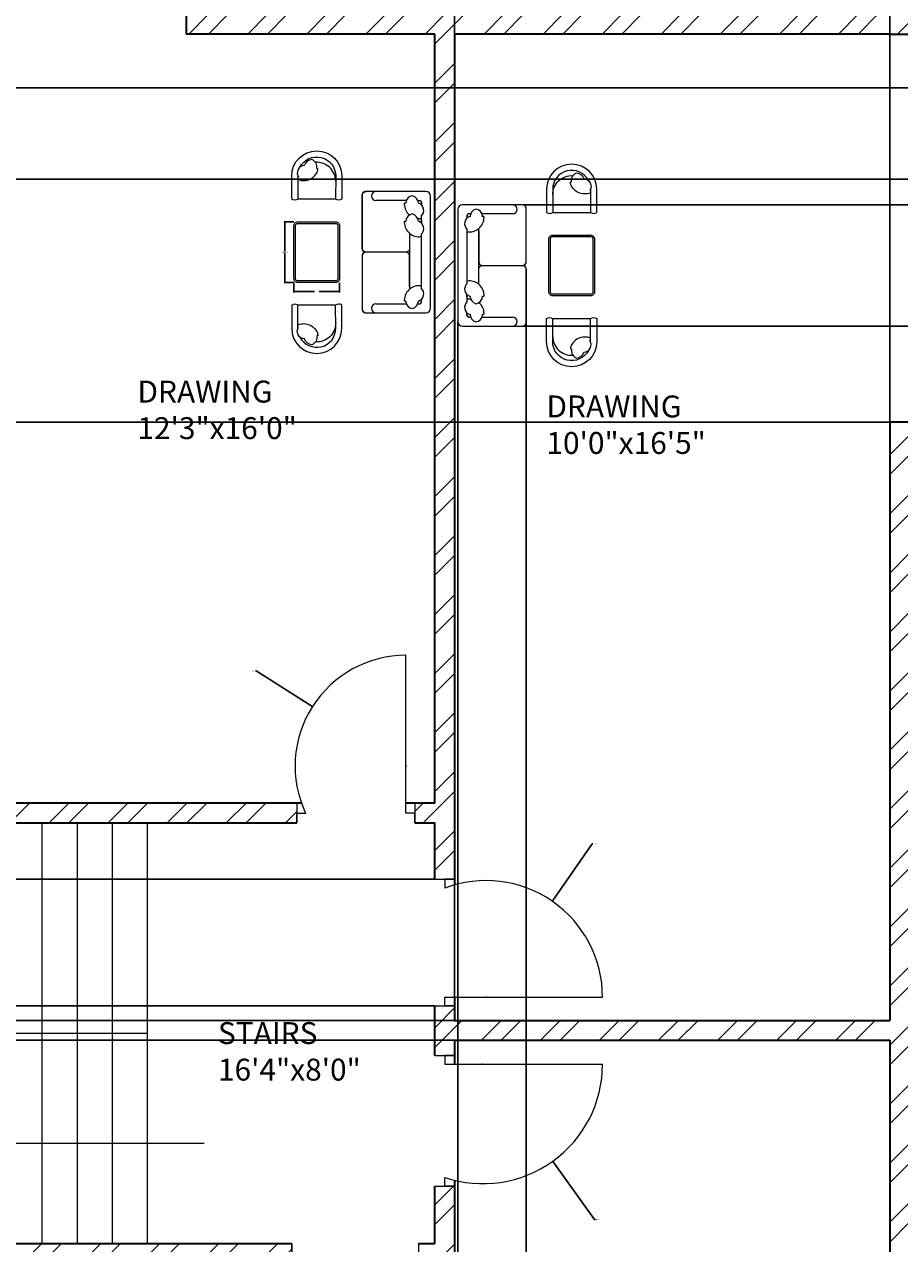
# Model space of a CAD drawing. Units: inches. Extents: x 2008 to 2657, y 1077 to 2165.
# Tile 9 of 16: x 2209 to 2409, y 1567 to 1845. Entities that reach past the tile are written whole.
import ezdxf

# ---------------------------------------------------------------- set-up
doc = ezdxf.new("R2010")
doc.units = ezdxf.units.IN
for name, color, linetype, lineweight in [('A-ANNO-DIMS', 2, 'Continuous', 18), ('A-AREA-IDEN', 4, 'Continuous', 18), ('A-DOOR', 11, 'Continuous', 18), ('A-FLOR-STRS', 60, 'Continuous', 18), ('A-FURN', 8, 'Continuous', 13), ('A-WALL', 7, 'Continuous', 35)]:
    doc.layers.add(name, color=color, linetype=linetype, lineweight=lineweight)
doc.layers.add('A-WALL-PATT', color=30, linetype='Continuous', lineweight=13, true_color=0xf8991e)
doc.styles.get("Standard").update_dxf_attribs({"font": 'arial.ttf'})
doc.dimstyles.get("Standard").update_dxf_attribs({"dimtxt": 0.18, "dimasz": 0.18, "dimexe": 0.18, "dimexo": 0.0625, "dimgap": 0.09, "dimtad": 0, "dimtih": 1, "dimtoh": 1, "dimdec": 4, "dimzin": 0, "dimdsep": 46, "dimtxsty": 'Standard', "dimcen": 0.09, "dimadec": 0, "dimazin": 0, "dimtfac": 1, "dimtdec": 4, "dimtofl": 0, "dimtmove": 0, "dimatfit": 3, "dimfxl": 1, "dimtolj": 1, "dimtzin": 0, "dimarcsym": 0})

# ---------------------------------------------------------------- blocks, each defined once
blk = doc.blocks.new('A$C1352')
at = {"color": 0}
for points in [[(0.003, 0.053), (0.003, 0.553, -0.414214), (0.053, 0.603), (0.753, 0.603, -0.414214), (0.803, 0.553), (0.803, 0.053, -0.414214), (0.753, 0.003), (0.053, 0.003, -0.414214)], [(0.023, 0.053), (0.023, 0.553, -0.414214), (0.053, 0.583), (0.753, 0.583, -0.414214), (0.783, 0.553), (0.783, 0.053, -0.414214), (0.753, 0.023), (0.053, 0.023, -0.414214)]]:
    blk.add_lwpolyline(points, format="xyb", close=True, dxfattribs=at)
blk = doc.blocks.new('LOUNGE-CHAIR')
blk.add_line((1.39, 5.54), (1.38, 0.26))
at = {"ltscale": 0.03}
blk.add_lwpolyline([(1.38, 0.26, -0.369229), (0, 0.27), (0, 5.54, -1), (11.42, 5.53), (11.42, 0.25, -0.369229), (10.03, 0.26)], format="xyb", close=True, dxfattribs=at)
blk.add_lwpolyline([(1.88, 7.54, -0.785087), (10.04, 5.53), (10.03, 0.26)], format="xyb")
for centre, radius, start, end in [((4.77, 7.34), 1.95, 94.9999, 161.3534), ((3.98, 7.61), 1.78, 346.6403, 69.4695), ((5.71, 4.32), 4.33, 359.9461, 93.658), ((3.01, 6.23), 1.73, 92.9922, 214.1401), ((5.71, 5.54), 4.33, 178.8536, 179.9461), ((2.75, 7.82), 3.35, 247.0143, 344.2857), ((5.79, 7.01), 0.207, 330.6238, 113.7423)]:
    blk.add_arc(centre, radius, start, end)
blk = doc.blocks.new('*D17')
at = {"layer": 'A-ANNO-DIMS', "color": 0, "lineweight": -2, "transparency": 16777216}
for p, q in [((2270.8, 1799.92), (2268.61, 1799.92)), ((2268.79, 1799.74), (2268.79, 1793.18)), ((2268.79, 1786.26), (2268.79, 1792.82)), ((2270.8, 1786.08), (2268.61, 1786.08))]:
    blk.add_line(p, q, dxfattribs=at)
at = {"layer": 'A-ANNO-DIMS', "color": 0, "transparency": 16777216}
for points in [[(2268.76, 1799.74), (2268.82, 1799.74), (2268.79, 1799.92)], [(2268.76, 1786.26), (2268.82, 1786.26), (2268.79, 1786.08)]]:
    blk.add_solid(points, dxfattribs=at)
at = {"layer": 'Defpoints', "color": 0, "transparency": 16777216}
for p in [(2270.87, 1799.92), (2268.79, 1786.08), (2270.87, 1786.08)]:
    blk.add_point(p, dxfattribs=at)
at = {"layer": 'A-ANNO-DIMS', "color": 0, "transparency": 16777216, "insert": (2268.79, 1793), "char_height": 0.18, "attachment_point": 5}
blk.add_mtext('\\A1;TABLE 14 TYP.', dxfattribs=at)
blk = doc.blocks.new('*D18')
at = {"layer": 'A-ANNO-DIMS', "color": 0, "lineweight": -2, "transparency": 16777216}
for p, q in [((2270.87, 1786.01), (2270.87, 1783.82)), ((2271.05, 1784), (2275.54, 1784)), ((2281.07, 1784), (2276.58, 1784)), ((2281.25, 1786.01), (2281.25, 1783.82))]:
    blk.add_line(p, q, dxfattribs=at)
at = {"layer": 'A-ANNO-DIMS', "color": 0, "transparency": 16777216}
for points in [[(2271.05, 1784.03), (2271.05, 1783.97), (2270.87, 1784)], [(2281.07, 1784.03), (2281.07, 1783.97), (2281.25, 1784)]]:
    blk.add_solid(points, dxfattribs=at)
at = {"layer": 'Defpoints', "color": 0, "transparency": 16777216}
for p in [(2270.87, 1786.08), (2281.25, 1786.08), (2281.25, 1784)]:
    blk.add_point(p, dxfattribs=at)
at = {"layer": 'A-ANNO-DIMS', "color": 0, "transparency": 16777216, "insert": (2276.06, 1784), "char_height": 0.18, "attachment_point": 5}
blk.add_mtext('\\A1;10 TYP.', dxfattribs=at)
blk = doc.blocks.new('*D51')
at = {"layer": 'A-ANNO-DIMS', "color": 0, "lineweight": -2, "transparency": 16777216}
for p, q in [((2307.5, 1617.74), (2307.5, 2142.9)), ((2307.68, 2142.72), (2356.74, 2142.72)), ((2406.58, 2142.72), (2357.53, 2142.72)), ((2406.76, 1617.74), (2406.76, 2142.9))]:
    blk.add_line(p, q, dxfattribs=at)
at = {"layer": 'A-ANNO-DIMS', "color": 0, "transparency": 16777216}
for points in [[(2307.68, 2142.75), (2307.68, 2142.69), (2307.5, 2142.72)], [(2406.58, 2142.75), (2406.58, 2142.69), (2406.76, 2142.72)]]:
    blk.add_solid(points, dxfattribs=at)
at = {"layer": 'Defpoints', "color": 0, "transparency": 16777216}
for p in [(2406.76, 2142.72), (2307.5, 1617.67), (2406.76, 1617.67)]:
    blk.add_point(p, dxfattribs=at)
at = {"layer": 'A-ANNO-DIMS', "color": 0, "transparency": 16777216, "insert": (2357.13, 2142.72), "char_height": 0.18, "attachment_point": 5}
blk.add_mtext('\\A1;99.26', dxfattribs=at)
blk = doc.blocks.new('*D52')
at = {"layer": 'A-ANNO-DIMS', "color": 0, "lineweight": -2, "transparency": 16777216}
for p, q in [((2406.7, 1754.17), (2028.03, 1754.17)), ((2028.21, 1753.99), (2028.21, 1686.11)), ((2028.21, 1617.85), (2028.21, 1685.74)), ((2406.7, 1617.67), (2028.03, 1617.67))]:
    blk.add_line(p, q, dxfattribs=at)
at = {"layer": 'A-ANNO-DIMS', "color": 0, "transparency": 16777216}
for points in [[(2028.18, 1753.99), (2028.24, 1753.99), (2028.21, 1754.17)], [(2028.18, 1617.85), (2028.24, 1617.85), (2028.21, 1617.67)]]:
    blk.add_solid(points, dxfattribs=at)
at = {"layer": 'Defpoints', "color": 0, "transparency": 16777216}
for p in [(2406.76, 1754.17), (2028.21, 1617.67), (2406.76, 1617.67)]:
    blk.add_point(p, dxfattribs=at)
at = {"layer": 'A-ANNO-DIMS', "color": 0, "transparency": 16777216, "insert": (2028.21, 1685.92), "char_height": 0.18, "attachment_point": 5}
blk.add_mtext('\\A1;136.5', dxfattribs=at)
blk = doc.blocks.new('*D53')
at = {"layer": 'A-ANNO-DIMS', "color": 0, "lineweight": -2, "transparency": 16777216}
for p, q in [((2406.7, 1613.17), (2028.03, 1613.17)), ((2028.21, 1612.99), (2028.21, 1545.11)), ((2028.21, 1476.85), (2028.21, 1544.74)), ((2406.7, 1476.67), (2028.03, 1476.67))]:
    blk.add_line(p, q, dxfattribs=at)
at = {"layer": 'A-ANNO-DIMS', "color": 0, "transparency": 16777216}
for points in [[(2028.18, 1612.99), (2028.24, 1612.99), (2028.21, 1613.17)], [(2028.18, 1476.85), (2028.24, 1476.85), (2028.21, 1476.67)]]:
    blk.add_solid(points, dxfattribs=at)
at = {"layer": 'Defpoints', "color": 0, "transparency": 16777216}
for p in [(2406.76, 1613.17), (2028.21, 1476.67), (2406.76, 1476.67)]:
    blk.add_point(p, dxfattribs=at)
at = {"layer": 'A-ANNO-DIMS', "color": 0, "transparency": 16777216, "insert": (2028.21, 1544.92), "char_height": 0.18, "attachment_point": 5}
blk.add_mtext('\\A1;136.5', dxfattribs=at)
blk = doc.blocks.new('*D58')
at = {"layer": 'A-ANNO-DIMS', "color": 0, "lineweight": -2, "transparency": 16777216}
for p, q in [((2459.7, 1830.5), (2028.03, 1830.5)), ((2028.21, 1830.32), (2028.21, 1820.26)), ((2028.21, 1809.84), (2028.21, 1819.9)), ((2459.7, 1809.66), (2028.03, 1809.66))]:
    blk.add_line(p, q, dxfattribs=at)
at = {"layer": 'A-ANNO-DIMS', "color": 0, "transparency": 16777216}
for points in [[(2028.18, 1830.32), (2028.24, 1830.32), (2028.21, 1830.5)], [(2028.18, 1809.84), (2028.24, 1809.84), (2028.21, 1809.66)]]:
    blk.add_solid(points, dxfattribs=at)
at = {"layer": 'Defpoints', "color": 0, "transparency": 16777216}
for p in [(2028.21, 1830.5), (2459.76, 1830.5), (2459.76, 1809.66)]:
    blk.add_point(p, dxfattribs=at)
at = {"layer": 'A-ANNO-DIMS', "color": 0, "transparency": 16777216, "insert": (2028.21, 1820.08), "char_height": 0.18, "attachment_point": 5}
blk.add_mtext('\\A1;20.835', dxfattribs=at)
blk = doc.blocks.new('*D59')
at = {"layer": 'A-ANNO-DIMS', "color": 0, "lineweight": -2, "transparency": 16777216}
for p, q in [((2302.94, 1649.88), (2028.03, 1649.88)), ((2028.21, 1649.7), (2028.21, 1635.62)), ((2028.21, 1621.18), (2028.21, 1635.26)), ((2302.94, 1621), (2028.03, 1621))]:
    blk.add_line(p, q, dxfattribs=at)
at = {"layer": 'A-ANNO-DIMS', "color": 0, "transparency": 16777216}
for points in [[(2028.18, 1649.7), (2028.24, 1649.7), (2028.21, 1649.88)], [(2028.18, 1621.18), (2028.24, 1621.18), (2028.21, 1621)]]:
    blk.add_solid(points, dxfattribs=at)
at = {"layer": 'Defpoints', "color": 0, "transparency": 16777216}
for p in [(2028.21, 1649.88), (2303, 1649.88), (2303, 1621)]:
    blk.add_point(p, dxfattribs=at)
at = {"layer": 'A-ANNO-DIMS', "color": 0, "transparency": 16777216, "insert": (2028.21, 1635.44), "char_height": 0.18, "attachment_point": 5}
blk.add_mtext('\\A1;28.875', dxfattribs=at)
blk = doc.blocks.new('*D64')
at = {"layer": 'A-ANNO-DIMS', "color": 0, "lineweight": -2, "transparency": 16777216}
for p, q in [((2308.25, 1777.08), (2308.25, 1140.44)), ((2323.83, 1776.91), (2323.83, 1140.44)), ((2308.43, 1140.62), (2315.59, 1140.62)), ((2323.65, 1140.62), (2316.49, 1140.62))]:
    blk.add_line(p, q, dxfattribs=at)
at = {"layer": 'A-ANNO-DIMS', "color": 0, "transparency": 16777216}
for points in [[(2308.43, 1140.65), (2308.43, 1140.59), (2308.25, 1140.62)], [(2323.65, 1140.65), (2323.65, 1140.59), (2323.83, 1140.62)]]:
    blk.add_solid(points, dxfattribs=at)
at = {"layer": 'Defpoints', "color": 0, "transparency": 16777216}
for p in [(2308.25, 1777.15), (2323.83, 1776.97), (2323.83, 1140.62)]:
    blk.add_point(p, dxfattribs=at)
at = {"layer": 'A-ANNO-DIMS', "color": 0, "transparency": 16777216, "insert": (2316.04, 1140.62), "char_height": 0.18, "attachment_point": 5}
blk.add_mtext('\\A1;15.572', dxfattribs=at)
blk = doc.blocks.new('*D65')
at = {"layer": 'A-ANNO-DIMS', "color": 0, "lineweight": -2, "transparency": 16777216}
for p, q in [((2323.2, 1803.79), (2624.99, 1803.79)), ((2624.81, 1803.61), (2624.81, 1790.13)), ((2624.81, 1776.29), (2624.81, 1789.77)), ((2323.2, 1776.11), (2624.99, 1776.11))]:
    blk.add_line(p, q, dxfattribs=at)
at = {"layer": 'A-ANNO-DIMS', "color": 0, "transparency": 16777216}
for points in [[(2624.78, 1803.61), (2624.84, 1803.61), (2624.81, 1803.79)], [(2624.78, 1776.29), (2624.84, 1776.29), (2624.81, 1776.11)]]:
    blk.add_solid(points, dxfattribs=at)
at = {"layer": 'Defpoints', "color": 0, "transparency": 16777216}
for p in [(2323.13, 1803.79), (2323.13, 1776.11), (2624.81, 1776.11)]:
    blk.add_point(p, dxfattribs=at)
at = {"layer": 'A-ANNO-DIMS', "color": 0, "transparency": 16777216, "insert": (2624.81, 1789.95), "char_height": 0.18, "attachment_point": 5}
blk.add_mtext('\\A1;27.684', dxfattribs=at)
blk = doc.blocks.new('*D76')
at = {"layer": 'A-ANNO-DIMS', "color": 0, "lineweight": -2, "transparency": 16777216}
for p, q in [((2313.88, 1607.69), (2314.06, 1607.69)), ((2313.97, 1607.6), (2313.97, 1607.78)), ((2339.43, 1572.24), (2329.99, 1585.39)), ((2339.61, 1572.24), (2339.43, 1572.24))]:
    blk.add_line(p, q, dxfattribs=at)
at = {"layer": 'A-ANNO-DIMS', "color": 0, "transparency": 16777216}
blk.add_solid([(2330.01, 1585.41), (2329.96, 1585.37), (2329.88, 1585.54)], dxfattribs=at)
at = {"layer": 'Defpoints', "color": 0, "transparency": 16777216}
for p in [(2313.97, 1607.69), (2329.88, 1585.54)]:
    blk.add_point(p, dxfattribs=at)
at = {"layer": 'A-ANNO-DIMS', "color": 0, "transparency": 16777216, "insert": (2340.09, 1572.24), "char_height": 0.18, "attachment_point": 5}
blk.add_mtext('\\A1;R27.28', dxfattribs=at)
blk = doc.blocks.new('*D77')
at = {"layer": 'A-ANNO-DIMS', "color": 0, "lineweight": -2, "transparency": 16777216}
for p, q in [((2338.85, 1658.01), (2329.88, 1645.03)), ((2339.03, 1658.01), (2338.85, 1658.01)), ((2314.57, 1623), (2314.75, 1623)), ((2314.66, 1622.91), (2314.66, 1623.09))]:
    blk.add_line(p, q, dxfattribs=at)
at = {"layer": 'A-ANNO-DIMS', "color": 0, "transparency": 16777216}
blk.add_solid([(2329.85, 1645.05), (2329.9, 1645.01), (2329.77, 1644.88)], dxfattribs=at)
at = {"layer": 'Defpoints', "color": 0, "transparency": 16777216}
for p in [(2329.77, 1644.88), (2314.66, 1623)]:
    blk.add_point(p, dxfattribs=at)
at = {"layer": 'A-ANNO-DIMS', "color": 0, "transparency": 16777216, "insert": (2339.57, 1658.01), "char_height": 0.18, "attachment_point": 5}
blk.add_mtext('\\A1;R26.594', dxfattribs=at)
blk = doc.blocks.new('*D81')
at = {"layer": 'A-ANNO-DIMS', "color": 0, "lineweight": -2, "transparency": 16777216}
for p, q in [((2262.1, 1697.43), (2262.28, 1697.43)), ((2262.28, 1697.43), (2274.93, 1689.38)), ((2296.33, 1675.69), (2296.51, 1675.69)), ((2296.42, 1675.6), (2296.42, 1675.78))]:
    blk.add_line(p, q, dxfattribs=at)
at = {"layer": 'A-ANNO-DIMS', "color": 0, "transparency": 16777216}
blk.add_solid([(2274.94, 1689.4), (2274.91, 1689.35), (2275.08, 1689.28)], dxfattribs=at)
at = {"layer": 'Defpoints', "color": 0, "transparency": 16777216}
for p in [(2275.08, 1689.28), (2296.42, 1675.69)]:
    blk.add_point(p, dxfattribs=at)
at = {"layer": 'A-ANNO-DIMS', "color": 0, "transparency": 16777216, "insert": (2261.69, 1697.43), "char_height": 0.18, "attachment_point": 5}
blk.add_mtext('\\A1;R25.3', dxfattribs=at)

msp = doc.modelspace()

# ---------------------------------------------------------------- hatches: boundary and pattern name
at = {"layer": 'A-WALL-PATT'}
h = msp.add_hatch(dxfattribs=at)
h.set_pattern_fill('ANSI32', color=256)
h.paths.add_polyline_path([(2109.2619, 2094.6743), (2104.7619, 2094.6743), (2104.7619, 2072.1743), (2104.7619, 2021.6151), (2109.2619, 2021.6151), (2109.2619, 2055.6743), (2126.1387, 2055.6743), (2126.1387, 2057.9243), (2126.1387, 2060.1743), (2109.2619, 2060.1743)])
h.paths.add_polyline_path([(2223.2494, 2057.9243), (2223.2494, 2060.1743), (2186.1387, 2060.1743), (2186.1387, 2055.6743), (2223.2494, 2055.6743)])
h.paths.add_polyline_path([(2250.7619, 2072.1743), (2250.7619, 2090.1743), (2250.7619, 2094.6743), (2246.2619, 2094.6743), (2246.2619, 2060.1743), (2242.7242, 2060.1743), (2242.7242, 2055.6743), (2246.2619, 2055.6743), (2246.2619, 1899.6743), (2242.7458, 1899.6743), (2242.7458, 1897.4243), (2242.7458, 1895.1743), (2246.2619, 1895.1743), (2246.2619, 1878.8745), (2248.5119, 1878.8745), (2250.7619, 1878.8745), (2250.7619, 1991.1743), (2250.7619, 2025.6743), (2257.6798, 2025.6743), (2257.6798, 2027.9243), (2257.6798, 2030.1743), (2250.7619, 2030.1743)])
h.paths.add_polyline_path([(2411.2619, 2031.6743), (2409.0119, 2031.6743), (2406.7619, 2031.6743), (2406.7619, 2030.1743), (2322.7619, 2030.1743), (2322.7619, 2053.3443), (2318.2619, 2053.3443), (2318.2619, 2030.1743), (2305.6798, 2030.1743), (2305.6798, 2025.6743), (2318.2619, 2025.6743), (2322.7619, 2025.6743), (2406.7619, 2025.6743), (2406.7619, 1995.6743), (2406.7619, 1847.2677), (2250.7619, 1847.2677), (2250.7619, 1850.9902), (2248.5119, 1850.9902), (2246.2619, 1850.9902), (2246.2619, 1847.1743), (2246.2619, 1842.7677), (2303.0015, 1842.7677), (2303.0015, 1667.2413), (2298.4208, 1667.2413), (2298.4208, 1662.7413), (2303.0015, 1662.7413), (2303.0015, 1649.8758), (2307.5015, 1649.8758), (2307.5015, 1842.7677), (2406.7619, 1842.7677), (2411.2619, 1842.7677), (2411.2619, 1878.6743), (2415.8196, 1878.6743), (2415.8196, 1880.9243), (2415.8196, 1883.1743), (2411.2619, 1883.1743)])
h.paths.add_polyline_path([(2411.2619, 2094.6743), (2406.7619, 2094.6743), (2318.2619, 2094.6743), (2318.2619, 2077.3443), (2322.7619, 2077.3443), (2322.7619, 2090.1743), (2406.7619, 2090.1743), (2406.7619, 2072.1743), (2406.7619, 2067.6743), (2406.7619, 2052.7524), (2411.2619, 2052.7524), (2411.2619, 2055.6743), (2414.9888, 2055.6743), (2414.9888, 2057.9243), (2414.9888, 2060.1743), (2411.2619, 2060.1743), (2411.2619, 2072.1743)])
h.paths.add_polyline_path([(2576.7619, 2072.1743), (2576.7619, 2094.6743), (2572.2619, 2094.6743), (2572.2619, 2060.1743), (2525.8113, 2060.1743), (2525.8113, 2055.6743), (2572.2619, 2055.6743), (2572.2619, 1994.289), (2576.7619, 1994.289)])
h.paths.add_polyline_path([(2465.8113, 2060.1743), (2436.2802, 2060.1743), (2436.2802, 2055.6743), (2465.8113, 2055.6743), (2465.8113, 2057.9243)])
h.paths.add_polyline_path([(2576.7619, 1934.289), (2574.5119, 1934.289), (2572.2619, 1934.289), (2572.2619, 1883.1743), (2447.7027, 1883.1743), (2447.7027, 1878.6743), (2459.7619, 1878.6743), (2459.7619, 1830.4982), (2464.2619, 1830.4982), (2464.2619, 1878.6743), (2572.2619, 1878.6743), (2572.2619, 1868.4883), (2576.7619, 1868.4883)])
h.paths.add_polyline_path([(2576.7619, 1832.4883), (2572.2619, 1832.4883), (2572.2619, 1806.6743), (2464.2619, 1806.6743), (2464.2619, 1809.6629), (2459.7619, 1809.6629), (2459.7619, 1802.1743), (2483.7619, 1802.1743), (2483.7619, 1778.1743), (2488.2619, 1778.1743), (2488.2619, 1802.1743), (2572.2619, 1802.1743), (2572.2619, 1793.6101), (2576.7619, 1793.6101)])
h.paths.add_polyline_path([(2576.7619, 1769.6101), (2572.2619, 1769.6101), (2572.2619, 1754.1743), (2488.2619, 1754.1743), (2488.2619, 1757.2675), (2486.0119, 1757.2675), (2483.7619, 1757.2675), (2483.7619, 1754.1743), (2447.4528, 1754.1743), (2447.4528, 1749.6743), (2483.7619, 1749.6743), (2572.2619, 1749.6743), (2572.2619, 1715.1837), (2576.7619, 1715.1837)])
h.paths.add_polyline_path([(2576.7619, 1655.1837), (2572.2619, 1655.1837), (2572.2619, 1617.6743), (2411.2619, 1617.6743), (2411.2619, 1749.6743), (2414.2827, 1749.6743), (2414.2827, 1754.1743), (2406.7619, 1754.1743), (2406.7619, 1749.6743), (2406.7619, 1617.6743), (2307.5015, 1617.6743), (2307.5015, 1621.0007), (2305.2515, 1621.0007), (2303.0015, 1621.0007), (2303.0015, 1609.6944), (2307.5015, 1609.6944), (2307.5015, 1613.1743), (2406.7619, 1613.1743), (2406.7619, 1476.6743), (2415.532, 1476.6743), (2415.532, 1478.9243), (2415.532, 1481.1743), (2411.2619, 1481.1743), (2411.2619, 1613.1743), (2572.2619, 1613.1743), (2572.2619, 1584.6086), (2576.7619, 1584.6086)])
h.paths.add_polyline_path([(2576.7619, 1524.6086), (2572.2619, 1524.6086), (2572.2619, 1481.1743), (2483.7619, 1481.1743), (2447.5119, 1481.1743), (2447.5119, 1476.6743), (2483.7619, 1476.6743), (2483.7619, 1473.5051), (2488.2619, 1473.5051), (2488.2619, 1476.6743), (2572.2619, 1476.6743), (2572.2619, 1469.5488), (2576.7619, 1469.5488)])
h.paths.add_polyline_path([(2576.7619, 1445.5488), (2572.2619, 1445.5488), (2572.2619, 1428.6743), (2488.2619, 1428.6743), (2488.2619, 1455.6743), (2486.0119, 1455.6743), (2483.7619, 1455.6743), (2483.7619, 1428.6743), (2459.7619, 1428.6743), (2459.7619, 1422.1519), (2464.2619, 1422.1519), (2464.2619, 1424.1743), (2572.2619, 1424.1743), (2572.2619, 1407.5685), (2576.7619, 1407.5685)])
h.paths.add_polyline_path([(2576.7619, 1371.5685), (2572.2619, 1371.5685), (2572.2619, 1352.1743), (2464.2619, 1352.1743), (2464.2619, 1403.1384), (2462.0119, 1403.1384), (2459.7619, 1403.1384), (2459.7619, 1352.1743), (2446.3194, 1352.1743), (2446.3194, 1347.6743), (2572.2619, 1347.6743), (2572.2619, 1321.0291), (2576.7619, 1321.0291)])
h.paths.add_polyline_path([(2462.703, 1227.6743), (2436.0298, 1227.6743), (2436.0298, 1225.4243), (2436.0298, 1223.1743), (2462.703, 1223.1743), (2462.703, 1225.4243)])
h.paths.add_polyline_path([(2576.7619, 1261.0291), (2574.5119, 1261.0291), (2572.2619, 1261.0291), (2572.2619, 1227.6743), (2522.703, 1227.6743), (2522.703, 1223.1743), (2572.2619, 1223.1743), (2572.2619, 1188.6743), (2576.7619, 1188.6743), (2576.7619, 1193.1743), (2576.7619, 1223.1743)])
h.paths.add_polyline_path([(2414.2823, 1227.6743), (2411.2619, 1227.6743), (2411.2619, 1267.1779), (2409.0119, 1267.1779), (2406.7619, 1267.1779), (2406.7619, 1227.6743), (2322.7619, 1227.6743), (2322.7619, 1244.3623), (2318.2619, 1244.3623), (2318.2619, 1223.1743), (2406.7619, 1223.1743), (2406.7619, 1193.1743), (2406.7619, 1188.6743), (2411.2619, 1188.6743), (2411.2619, 1193.1743), (2411.2619, 1223.1743), (2414.2823, 1223.1743)])
h.paths.add_polyline_path([(2411.2619, 1347.6743), (2414.702, 1347.6743), (2414.702, 1349.9243), (2414.702, 1352.1743), (2411.2619, 1352.1743), (2411.2619, 1416.7413), (2307.5015, 1416.7413), (2307.5015, 1579.8489), (2305.2515, 1579.8489), (2303.0015, 1579.8489), (2303.0015, 1566.7413), (2299.2719, 1566.7413), (2299.2719, 1562.2413), (2303.0015, 1562.2413), (2303.0015, 1416.7413), (2246.2619, 1416.7413), (2246.2619, 1409.8616), (2250.7619, 1409.8616), (2250.7619, 1412.2413), (2406.7619, 1412.2413), (2406.7619, 1292.1743), (2304.9703, 1292.1743), (2304.9703, 1287.6743), (2318.2619, 1287.6743), (2318.2619, 1268.3623), (2322.7619, 1268.3623), (2322.7619, 1287.6743), (2406.7619, 1287.6743), (2406.7619, 1285.4748), (2411.2619, 1285.4748)])
h.paths.add_polyline_path([(2109.2619, 1262.7482), (2104.7619, 1262.7482), (2104.7619, 1223.1743), (2104.7619, 1193.1743), (2104.7619, 1188.6743), (2109.2619, 1188.6743), (2109.2619, 1223.1743), (2126.7928, 1223.1743), (2126.7928, 1225.4243), (2126.7928, 1227.6743), (2109.2619, 1227.6743)])
h.paths.add_polyline_path([(2222.3268, 1227.6743), (2186.7928, 1227.6743), (2186.7928, 1223.1743), (2222.3268, 1223.1743)])
h.paths.add_polyline_path([(2250.7619, 1287.6743), (2256.9703, 1287.6743), (2256.9703, 1289.9243), (2256.9703, 1292.1743), (2250.7619, 1292.1743), (2250.7619, 1382.2078), (2248.5119, 1382.2078), (2246.2619, 1382.2078), (2246.2619, 1347.6743), (2246.2619, 1227.6743), (2242.6068, 1227.6743), (2242.6068, 1223.1743), (2246.2619, 1223.1743), (2246.2619, 1188.6743), (2250.7619, 1188.6743), (2250.7619, 1193.1743), (2250.7619, 1227.6743)])
h.paths.add_polyline_path([(2133.2619, 1349.9243), (2133.2619, 1352.1743), (2109.2619, 1352.1743), (2109.2619, 1375.2826), (2104.7619, 1375.2826), (2104.7619, 1322.7482), (2109.2619, 1322.7482), (2109.2619, 1347.6743), (2133.2619, 1347.6743)])
h.paths.add_polyline_path([(2210.2105, 1352.1743), (2161.7619, 1352.1743), (2161.7619, 1412.2413), (2185.7619, 1412.2413), (2185.7619, 1420.1851), (2183.5119, 1420.1851), (2181.2619, 1420.1851), (2181.2619, 1416.7413), (2109.2619, 1416.7413), (2109.2619, 1452.4006), (2104.7619, 1452.4006), (2104.7619, 1399.2826), (2109.2619, 1399.2826), (2109.2619, 1412.2413), (2157.2619, 1412.2413), (2157.2619, 1352.1743), (2154.3383, 1352.1743), (2154.3383, 1347.6743), (2210.2105, 1347.6743)])
h.paths.add_polyline_path([(2185.7619, 1514.2413), (2161.7619, 1514.2413), (2161.7619, 1518.1307), (2159.5119, 1518.1307), (2157.2619, 1518.1307), (2157.2619, 1514.2413), (2109.2619, 1514.2413), (2109.2619, 1528.997), (2107.0119, 1528.997), (2104.7619, 1528.997), (2104.7619, 1488.4006), (2109.2619, 1488.4006), (2109.2619, 1509.7413), (2181.2619, 1509.7413), (2181.2619, 1441.2042), (2185.7619, 1441.2042)])
h.paths.add_polyline_path([(2270.4025, 1566.7413), (2109.2619, 1566.7413), (2080.7619, 1566.7413), (2080.7619, 1586.5643), (2076.2619, 1586.5643), (2076.2619, 1562.2413), (2080.7619, 1562.2413), (2104.7619, 1562.2413), (2104.7619, 1552.997), (2109.2619, 1552.997), (2109.2619, 1562.2413), (2157.2619, 1562.2413), (2157.2619, 1538.2413), (2161.7619, 1538.2413), (2161.7619, 1562.2413), (2205.2619, 1562.2413), (2270.4025, 1562.2413)])
h.paths.add_polyline_path([(2131.6813, 1897.4243), (2131.6813, 1899.6743), (2109.2619, 1899.6743), (2109.2619, 1961.6151), (2104.7619, 1961.6151), (2104.7619, 1886.8042), (2109.2619, 1886.8042), (2109.2619, 1895.1743), (2131.6813, 1895.1743)])
h.paths.add_polyline_path([(2185.7619, 1847.1743), (2161.7619, 1847.1743), (2161.7619, 1895.1743), (2185.7619, 1895.1743), (2211.543, 1895.1743), (2211.543, 1897.4243), (2211.543, 1899.6743), (2154.0916, 1899.6743), (2154.0916, 1897.4243), (2154.0916, 1895.1743), (2157.2619, 1895.1743), (2157.2619, 1847.1743), (2109.2619, 1847.1743), (2109.2619, 1862.8042), (2104.7619, 1862.8042), (2104.7619, 1821.243), (2109.2619, 1821.243), (2109.2619, 1842.6743), (2181.2619, 1842.6743), (2181.2619, 1840.6763), (2185.7619, 1840.6763)])
h.paths.add_polyline_path([(2109.2619, 1785.243), (2104.7619, 1785.243), (2104.7619, 1715.4691), (2109.2619, 1715.4691), (2109.2619, 1730.8423), (2157.2619, 1730.8423), (2157.2619, 1727.6404), (2161.7619, 1727.6404), (2161.7619, 1730.8423), (2185.7619, 1730.8423), (2185.7619, 1822.1438), (2183.5119, 1822.1438), (2181.2619, 1822.1438), (2181.2619, 1735.3423), (2109.2619, 1735.3423)])
h.paths.add_polyline_path([(2109.2619, 1691.4691), (2104.7619, 1691.4691), (2104.7619, 1667.2413), (2076.2619, 1667.2413), (2076.2619, 1646.5643), (2080.7619, 1646.5643), (2080.7619, 1662.7413), (2109.2619, 1662.7413), (2271.4941, 1662.7413), (2271.4941, 1664.9913), (2271.4941, 1667.2413), (2181.2619, 1667.2413), (2161.7619, 1667.2413), (2161.7619, 1708.3752), (2159.5119, 1708.3752), (2157.2619, 1708.3752), (2157.2619, 1667.2413), (2109.2619, 1667.2413)])
h.paths.add_polyline_path([(2233.1467, 1747.4973), (2270.0737, 1747.4973), (2270.0737, 1766.1547), (2233.1467, 1766.1547)], flags=9)

# ---------------------------------------------------------------- linework, layer by layer
at = {"layer": 'A-DOOR'}
for p, q in [((2296.4208, 1664.9913), (2296.4208, 1700.9913)), ((2271.4941, 1667.2413), (2271.4941, 1662.7413)), ((2298.4208, 1667.2413), (2298.4208, 1662.7413)), ((2271.4941, 1662.7413), (2271.4941, 1664.9913)), ((2271.4941, 1664.9913), (2273.4941, 1664.9913)), ((2298.4208, 1664.9913), (2296.4208, 1664.9913)), ((2298.4208, 1662.7413), (2298.4208, 1664.9913)), ((2303.0015, 1649.8758), (2307.5015, 1649.8758)), ((2307.5015, 1649.8758), (2305.2515, 1649.8758)), ((2305.2515, 1649.8758), (2305.2515, 1647.8758)), ((2305.2515, 1621.0007), (2305.2515, 1623.0007)), ((2305.2515, 1623.0007), (2341.2515, 1623.0007)), ((2303.0015, 1621.0007), (2307.5015, 1621.0007)), ((2307.5015, 1621.0007), (2305.2515, 1621.0007)), ((2303.0015, 1609.6944), (2307.5015, 1609.6944)), ((2307.5015, 1609.6944), (2305.2515, 1609.6944)), ((2305.2515, 1609.6944), (2305.2515, 1607.6944)), ((2305.2515, 1607.6944), (2341.2515, 1607.6944)), ((2305.2515, 1579.8489), (2305.2515, 1581.8489)), ((2303.0015, 1579.8489), (2307.5015, 1579.8489)), ((2307.5015, 1579.8489), (2305.2515, 1579.8489)), ((2270.4025, 1562.2413), (2270.4025, 1566.7413)), ((2270.4025, 1566.7413), (2270.4025, 1564.4913)), ((2299.2719, 1566.7413), (2299.2719, 1562.2413))]:
    msp.add_line(p, q, dxfattribs=at)
for centre, radius, start, end in [((2296.4208, 1675.6909), 25.3004, 90, 205.017851), ((2314.6575, 1623.0007), 26.5941, 0, 110.712894), ((2313.9739, 1607.6944), 27.2777, 251.35154, 0)]:
    msp.add_arc(centre, radius, start, end, dxfattribs=at)
at = {"layer": 'A-FLOR-STRS'}
for p, q in [((2213.3789, 1662.7413), (2213.3789, 1566.7413)), ((2221.3789, 1662.7413), (2221.3789, 1566.7413)), ((2229.3789, 1662.7413), (2229.3789, 1566.7413)), ((2237.3789, 1662.7413), (2237.3789, 1566.7413)), ((2117.3789, 1614.7413), (2237.3789, 1614.7413)), ((2250.4174, 1589.6092), (2096.9521, 1589.6092))]:
    msp.add_line(p, q, dxfattribs=at)
at = {"layer": 'A-FURN'}
for p, q in [((2296.4804, 1804.764), (2289.5533, 1804.764)), ((2299.107, 1804.764), (2299.5888, 1804.764)), ((2299.9348, 1804.4179), (2299.9348, 1803.7813)), ((2299.9348, 1799.6271), (2299.9348, 1801.2831)), ((2299.9348, 1800.2638), (2299.9348, 1799.6271)), ((2310.3296, 1801.3701), (2310.3296, 1800.7335)), ((2311.1575, 1801.7161), (2310.6757, 1801.7161)), ((2320.7111, 1801.7161), (2313.784, 1801.7161)), ((2310.3296, 1798.2353), (2310.3296, 1785.8197)), ((2299.9348, 1784.7134), (2299.9348, 1797.129)), ((2289.5533, 1781.2326), (2296.4804, 1781.2326)), ((2299.107, 1781.2326), (2299.5888, 1781.2326)), ((2299.9348, 1781.5786), (2299.9348, 1782.2152)), ((2310.3296, 1782.6849), (2310.3296, 1783.3215)), ((2310.3296, 1783.3215), (2310.3296, 1781.6656)), ((2310.3296, 1778.5308), (2310.3296, 1779.1674)), ((2311.1575, 1778.1847), (2310.6757, 1778.1847)), ((2313.784, 1778.1847), (2320.7111, 1778.1847))]:
    msp.add_line(p, q, dxfattribs=at)
at = {"layer": 'A-FURN', "ltscale": 0.03}
for points in [[(2287.131, 1792.9898, 0.41421356), (2286.4389, 1792.2977), (2286.4389, 1779.8483, 0.41421356), (2287.131, 1779.1562), (2300.973, 1779.1562, 0.41421356), (2302.0111, 1780.1944), (2302.0111, 1805.8021, 0.41421356), (2300.973, 1806.8403), (2287.131, 1806.8403, 0.41421356), (2286.4389, 1806.1482), (2286.4389, 1793.6989, 0.41421356), (2287.131, 1793.0068)], [(2323.1335, 1789.9589, 0.41421356), (2323.8256, 1790.651), (2323.8256, 1803.1003, 0.41421356), (2323.1335, 1803.7924), (2309.2915, 1803.7924, 0.41421356), (2308.2533, 1802.7543), (2308.2533, 1777.1466, 0.41421356), (2309.2915, 1776.1084), (2323.1335, 1776.1084, 0.41421356), (2323.8256, 1776.8005), (2323.8256, 1789.2498, 0.41421356), (2323.1335, 1789.9419)]]:
    msp.add_lwpolyline(points, format="xyb", dxfattribs=at)
at = {"layer": 'A-FURN'}
for points in [[(2297.2529, 1797.2678), (2297.2529, 1793.8634, -0.41421356), (2296.3878, 1792.9983), (2287.304, 1792.9983, -0.41421356), (2286.4389, 1793.8634), (2286.4389, 1805.9751, -0.41421356), (2287.304, 1806.8403)], [(2313.0115, 1797.7849), (2313.0115, 1790.8156, 0.41421356), (2313.8767, 1789.9504), (2322.9605, 1789.9504, 0.41421356), (2323.8256, 1790.8156), (2323.8256, 1802.9273, 0.41421356), (2322.9605, 1803.7924)], [(2297.2529, 1785.1638), (2297.2529, 1792.1331, 0.41421356), (2296.3878, 1792.9983), (2287.304, 1792.9983, 0.41421356), (2286.4389, 1792.1331), (2286.4389, 1780.0214, 0.41421356), (2287.304, 1779.1562)], [(2313.0115, 1785.6809), (2313.0115, 1789.0853, -0.41421356), (2313.8767, 1789.9504), (2322.9605, 1789.9504, -0.41421356), (2323.8256, 1789.0853), (2323.8256, 1776.9735, -0.41421356), (2322.9605, 1776.1084)]]:
    msp.add_lwpolyline(points, format="xyb", dxfattribs=at)
for points in [[(2313.0115, 1785.6809), (2313.0115, 1798.3741)], [(2297.2529, 1797.2678), (2297.2529, 1784.5745)]]:
    msp.add_lwpolyline(points, dxfattribs=at)
for centre, radius, start, end in [((2289.5533, 1805.8021), 1.0382, 90, 180), ((2289.5533, 1805.8021), 1.0382, 180, 270), ((2298.1346, 1804.1117), 1.7781, 96.427858, 179.256998), ((2297.2969, 1804.0347), 1.9514, 4.543938, 70.89739), ((2296.2297, 1803.9713), 0.207, 52.154994, 195.27353), ((2299.3783, 1804.011), 3.3497, 181.611631, 229.375991), ((2298.7326, 1802.5322), 1.7337, 311.757236, 72.905096), ((2299.5888, 1804.4179), 0.3461, 0, 90), ((2299.5888, 1804.4179), 0.3461, 0, 90), ((2320.7111, 1802.7543), 1.0382, 0, 90), ((2298.1346, 1799.9576), 1.7781, 96.427858, 179.256998), ((2297.2969, 1799.8805), 1.9514, 4.543938, 70.89739), ((2299.3783, 1804.011), 3.3497, 264.880983, 278.88305), ((2311.5319, 1799.4844), 1.7337, 107.094904, 228.242764), ((2310.6757, 1801.3701), 0.3461, 90, 180), ((2310.8862, 1800.9632), 3.3497, 261.11695, 358.388369), ((2312.9676, 1800.9868), 1.9514, 109.10261, 175.456062), ((2312.1299, 1801.0639), 1.7781, 0.743002, 83.572142), ((2314.0348, 1800.9235), 0.207, 344.72647, 127.845006), ((2320.7111, 1802.7543), 1.0382, 270, 0), ((2296.2297, 1799.8172), 0.207, 52.154994, 195.27353), ((2299.3783, 1799.8568), 3.3497, 181.611631, 278.88305), ((2298.7326, 1798.378), 1.7337, 311.757236, 72.905096), ((2310.8862, 1783.0918), 3.3497, 1.611631, 98.88305), ((2299.3783, 1781.9855), 3.3497, 81.11695, 178.388369), ((2298.7326, 1783.4643), 1.7337, 287.094904, 48.242764), ((2311.5319, 1784.5706), 1.7337, 131.757236, 252.905096), ((2289.5533, 1780.1944), 1.0382, 90, 180), ((2296.2297, 1782.0252), 0.207, 164.72647, 307.845006), ((2298.1346, 1781.8848), 1.7781, 180.743002, 263.572142), ((2297.2969, 1781.9618), 1.9514, 289.10261, 355.456062), ((2299.5888, 1781.5786), 0.3461, 270, 0), ((2311.5319, 1780.4165), 1.7337, 131.757236, 252.905096), ((2310.8862, 1778.9377), 3.3497, 84.880983, 98.88305), ((2312.9676, 1783.0682), 1.9514, 184.543938, 250.89739), ((2312.1299, 1782.9911), 1.7781, 276.427858, 359.256998), ((2310.8862, 1778.9377), 3.3497, 1.611631, 49.375991), ((2314.0348, 1783.1315), 0.207, 232.154994, 15.27353), ((2289.5533, 1780.1944), 1.0382, 180, 270), ((2310.6757, 1778.5308), 0.3461, 180, 270), ((2310.6757, 1778.5308), 0.3461, 180, 270), ((2312.9676, 1778.914), 1.9514, 184.543938, 250.89739), ((2312.1299, 1778.837), 1.7781, 276.427858, 359.256998), ((2314.0348, 1778.9774), 0.207, 232.154994, 15.27353), ((2320.7111, 1777.1466), 1.0382, 0, 90), ((2320.7111, 1777.1466), 1.0382, 270, 0)]:
    msp.add_arc(centre, radius, start, end, dxfattribs=at)
at = {"layer": 'A-WALL'}
for p, q in [((2246.2619, 1847.1743), (2246.2619, 1842.7677)), ((2303.0015, 1842.7677), (2246.2619, 1842.7677)), ((2303.0015, 1667.2413), (2303.0015, 1842.7677)), ((2406.7619, 1842.7677), (2307.5015, 1842.7677)), ((2307.5015, 1842.7677), (2307.5015, 1648.6139)), ((2406.7619, 1842.7677), (2411.2619, 1842.7677)), ((2406.7619, 1754.1743), (2406.7619, 1749.6743)), ((2406.7619, 1754.1743), (2406.7619, 1617.6743)), ((2414.2827, 1754.1743), (2406.7619, 1754.1743)), ((2272.573, 1667.2413), (2181.2619, 1667.2413)), ((2303.0015, 1667.2413), (2296.4208, 1667.2413)), ((2109.2619, 1662.7413), (2271.4941, 1662.7413)), ((2298.4208, 1662.7413), (2303.0015, 1662.7413)), ((2303.0015, 1649.8758), (2303.0015, 1662.7413)), ((2307.5015, 1623.0007), (2307.5015, 1617.6743)), ((2303.0015, 1609.6944), (2303.0015, 1621.0007)), ((2307.5015, 1617.6743), (2406.7619, 1617.6743)), ((2307.5015, 1613.1743), (2406.7619, 1613.1743)), ((2307.5015, 1613.1743), (2307.5015, 1607.6944)), ((2406.7619, 1613.1743), (2406.7619, 1476.6743)), ((2307.5015, 1581.1958), (2307.5015, 1416.7413)), ((2303.0015, 1566.7413), (2303.0015, 1579.8489)), ((2109.2619, 1566.7413), (2270.4025, 1566.7413)), ((2299.2719, 1566.7413), (2303.0015, 1566.7413))]:
    msp.add_line(p, q, dxfattribs=at)

# ---------------------------------------------------------------- block references
at = {"layer": 'A-FURN'}
msp.add_blockref('LOUNGE-CHAIR', (2270.348, 1804.85), dxfattribs=at)
at = {"layer": 'A-FURN', "extrusion": (0, 0, -1), "zscale": -1}
msp.add_blockref('LOUNGE-CHAIR', (-2339.9165, 1801.8022), dxfattribs=at)
at = {"layer": 'A-FURN', "ltscale": 0.03, "xscale": 17.30251319894821, "yscale": 17.30251319894821, "zscale": 17.30251319894821}
for p, rotation in [((2270.8148, 1799.9658), 270), ((2339.4497, 1782.9829), 89.99999999999999)]:
    msp.add_blockref('A$C1352', p, dxfattribs=dict(at, rotation=rotation))
at = {"layer": 'A-FURN', "extrusion": (0, 0, -1), "zscale": -1, "rotation": 180}
msp.add_blockref('LOUNGE-CHAIR', (-2270.348, 1781.1465), dxfattribs=at)
at = {"layer": 'A-FURN', "rotation": 180}
msp.add_blockref('LOUNGE-CHAIR', (2339.9165, 1778.0987), dxfattribs=at)

# ---------------------------------------------------------------- texts
at = {"layer": 'A-AREA-IDEN', "char_height": 5, "attachment_point": 1}
for s, width, insert in [('DRAWING\\P12\'3"x16\'0"', 109.233856, (2235.1572, 1763.6666)), ('DRAWING\\P10\'0"x16\'5"', 87.48756, (2328.4472, 1760.2845)), ('STAIRS\\P16\'4"x8\'0"', 110.131657, (2253.5238, 1617.2803))]:
    msp.add_mtext_dynamic_manual_height_columns(s, width=width, gutter_width=12.5, heights=[0], dxfattribs=dict(at, insert=insert))

# ---------------------------------------------------------------- dimensions: what is measured, and where the dimension line sits
at = {"layer": 'A-ANNO-DIMS'}
for base, p1, p2, override, picture, middle in [((2406.7619, 2142.7243), (2307.5015, 1617.6743), (2406.7619, 1617.6743), {"dimdec": 2, "dimlfac": 1, "dimrnd": 0, "dimzin": 0, "dimdsep": 46, "dimlunit": 2}, '*D51', (2357.1317, 2142.7243)), ((2323.8256, 1140.6243), (2308.2533, 1777.1466), (2323.8256, 1776.9735), {"dimdec": 3, "dimlfac": 1, "dimrnd": 0, "dimzin": 0, "dimdsep": 46, "dimlunit": 2}, '*D64', (2316.0395, 1140.6243))]:
    dim = msp.add_linear_dim(base=base, p1=p1, p2=p2, dimstyle='Standard', override=override, dxfattribs=at)
    dim.commit()
    dim.dimension.update_dxf_attribs({"geometry": picture, "text_midpoint": middle})
for base, p1, p2, override, picture, middle in [((2028.2119, 1830.4982), (2459.7619, 1809.6629), (2459.7619, 1830.4982), {"dimdec": 3, "dimlfac": 1, "dimrnd": 0, "dimzin": 0, "dimdsep": 46, "dimlunit": 2}, '*D58', (2028.2119, 1820.0806)), ((2624.8119, 1776.1084), (2323.1335, 1803.7924), (2323.1335, 1776.1084), {"dimdec": 3, "dimlfac": 1, "dimrnd": 0, "dimzin": 0, "dimdsep": 46, "dimlunit": 2}, '*D65', (2624.8119, 1789.9504)), ((2028.2119, 1617.6743), (2406.7619, 1754.1743), (2406.7619, 1617.6743), {"dimdec": 1, "dimlfac": 1, "dimrnd": 0, "dimzin": 0, "dimdsep": 46, "dimlunit": 2}, '*D52', (2028.2119, 1685.9243)), ((2028.2119, 1649.8758), (2303.0015, 1621.0007), (2303.0015, 1649.8758), {"dimdec": 3, "dimlfac": 1, "dimrnd": 0, "dimzin": 0, "dimdsep": 46, "dimlunit": 2}, '*D59', (2028.2119, 1635.4382)), ((2028.2119, 1476.6743), (2406.7619, 1613.1743), (2406.7619, 1476.6743), {"dimdec": 1, "dimlfac": 1, "dimrnd": 0, "dimzin": 0, "dimdsep": 46, "dimlunit": 2}, '*D53', (2028.2119, 1544.9243))]:
    dim = msp.add_linear_dim(base=base, p1=p1, p2=p2, angle=90, dimstyle='Standard', override=override, dxfattribs=at)
    dim.commit()
    dim.dimension.update_dxf_attribs({"geometry": picture, "text_midpoint": middle})
dim = msp.add_linear_dim(base=(2268.7903, 1786.0773), p1=(2270.8666, 1799.9193), p2=(2270.8666, 1786.0773), angle=270, text='TABLE <> TYP.', dimstyle='Standard', override={"dimdec": 0, "dimlfac": 1, "dimrnd": 0, "dimzin": 0, "dimdsep": 46, "dimlunit": 2}, dxfattribs=at)
dim.commit()
dim.dimension.update_dxf_attribs({"geometry": '*D17', "text_midpoint": (2268.7903, 1792.9983)})
dim = msp.add_linear_dim(base=(2281.2481, 1784.001), p1=(2270.8666, 1786.0773), p2=(2281.2481, 1786.0773), text='<> TYP.', dimstyle='Standard', override={"dimdec": 0, "dimlfac": 1, "dimrnd": 0, "dimzin": 0, "dimdsep": 46, "dimlunit": 2}, dxfattribs=at)
dim.commit()
dim.dimension.update_dxf_attribs({"geometry": '*D18', "text_midpoint": (2276.0574, 1784.001)})
for center, mpoint, override, picture, middle in [((2296.4208, 1675.6909), (2275.0801, 1689.2809), {"dimdec": 1, "dimlfac": 1, "dimrnd": 0, "dimzin": 0, "dimdsep": 46, "dimlunit": 2}, '*D81', (2261.6858, 1697.4349)), ((2314.6575, 1623.0007), (2329.775, 1644.88), {"dimdec": 3, "dimlfac": 1, "dimrnd": 0, "dimzin": 0, "dimdsep": 46, "dimlunit": 2}, '*D77', (2339.5749, 1658.0076)), ((2313.9739, 1607.6944), (2329.8821, 1585.5359), {"dimdec": 2, "dimlfac": 1, "dimrnd": 0, "dimzin": 0, "dimdsep": 46, "dimlunit": 2}, '*D76', (2340.087, 1572.2408))]:
    dim = msp.add_radius_dim(center=center, mpoint=mpoint, dimstyle='Standard', override=override, dxfattribs=at)
    dim.commit()
    dim.dimension.update_dxf_attribs({"geometry": picture, "text_midpoint": middle, "dimtype": 164})

doc.saveas('drawing.dxf')
